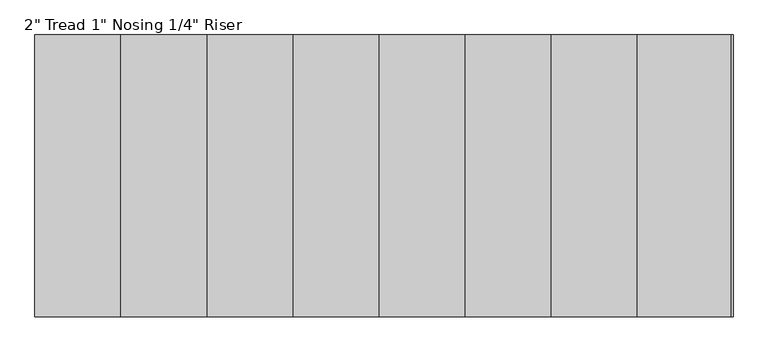
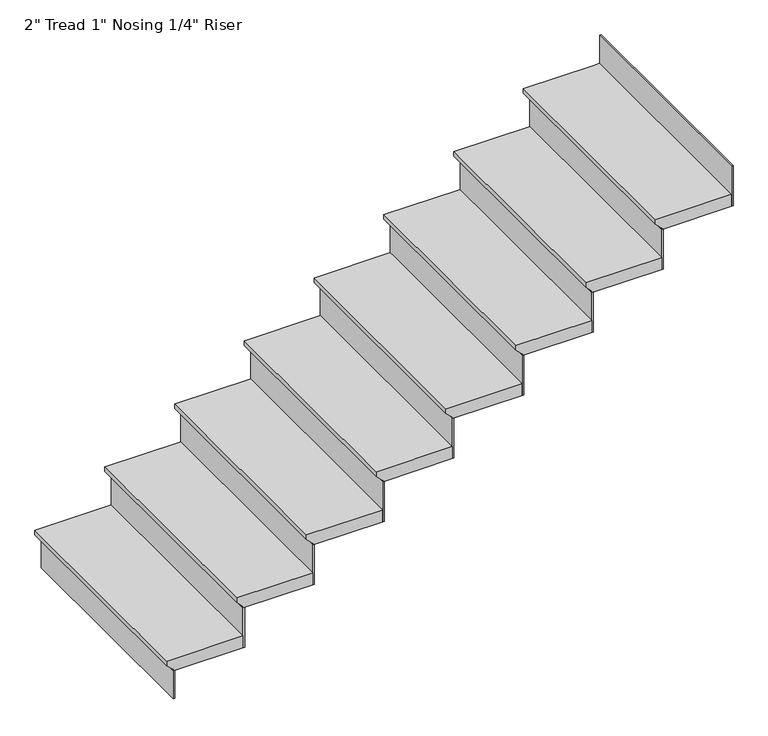
"""IFC4 building model written with IfcOpenShell, lengths in millimetres: stair flight geometry."""

from ifc_helpers import new_model, si_unit, origin, place, context, project, spatial, faceted_brep, source, transform, mapped, element, save


def stair_flight_5af034e0(model_context):
    return source(origin(), model_context, "Body", "Brep", [
        faceted_brep([(-4412.1017807, 444.1428136, 3350.6833333), (-4412.1017807, 444.1428136, 3369.7333333), (-4412.1017807, 1358.5428136, 3369.7333333), (-4412.1017807, 1358.5428136, 3350.6833333), (-4386.7017807, 444.1428136, 3325.2833333), (-4386.7017807, 1358.5428136, 3325.2833333), (-4107.3017807, 444.1428136, 3369.7333333), (-4107.3017807, 1358.5428136, 3369.7333333), (-4386.7017807, 1358.5428136, 3318.9333333), (-4107.3017807, 1358.5428136, 3318.9333333), (-4107.3017807, 444.1428136, 3318.9333333), (-4386.7017807, 444.1428136, 3318.9333333)], [[[0, 1, 2, 3]], [[4, 0, 3, 5]], [[2, 1, 6, 7]], [[8, 9, 10, 11]], [[2, 7, 9, 8, 5, 3]], [[8, 11, 4, 5]], [[6, 1, 0, 4, 11, 10]], [[7, 6, 10, 9]]]),
        faceted_brep([(-4386.7017807, 444.1428136, 3318.9333333), (-4386.7017807, 444.1428136, 3200.4), (-4380.3517807, 444.1428136, 3200.4), (-4380.3517807, 444.1428136, 3318.9333333), (-4386.7017807, 1358.5428136, 3318.9333333), (-4380.3517807, 1358.5428136, 3318.9333333), (-4380.3517807, 1358.5428136, 3200.4), (-4386.7017807, 1358.5428136, 3200.4)], [[[0, 1, 2, 3]], [[4, 5, 6, 7]], [[1, 0, 4, 7]], [[2, 1, 7, 6]], [[3, 2, 6, 5]], [[0, 3, 5, 4]]]),
        faceted_brep([(-4107.3017807, 444.1428136, 3488.2666667), (-4107.3017807, 444.1428136, 3318.9333333), (-4100.9517807, 444.1428136, 3318.9333333), (-4100.9517807, 444.1428136, 3488.2666667), (-4107.3017807, 1358.5428136, 3488.2666667), (-4100.9517807, 1358.5428136, 3488.2666667), (-4100.9517807, 1358.5428136, 3318.9333333), (-4107.3017807, 1358.5428136, 3318.9333333)], [[[0, 1, 2, 3]], [[4, 5, 6, 7]], [[1, 0, 4, 7]], [[2, 1, 7, 6]], [[3, 2, 6, 5]], [[0, 3, 5, 4]]]),
        faceted_brep([(-4132.7017807, 1358.5428136, 3539.0666667), (-4132.7017807, 444.1428136, 3539.0666667), (-3827.9017807, 444.1428136, 3539.0666667), (-3827.9017807, 1358.5428136, 3539.0666667), (-4107.3017807, 1358.5428136, 3488.2666667), (-3827.9017807, 1358.5428136, 3488.2666667), (-3827.9017807, 444.1428136, 3488.2666667), (-4107.3017807, 444.1428136, 3488.2666667), (-4107.3017807, 1358.5428136, 3494.6166667), (-4132.7017807, 1358.5428136, 3520.0166667), (-4107.3017807, 444.1428136, 3494.6166667), (-4132.7017807, 444.1428136, 3520.0166667)], [[[0, 1, 2, 3]], [[4, 5, 6, 7]], [[0, 3, 5, 4, 8, 9]], [[4, 7, 10, 8]], [[2, 1, 11, 10, 7, 6]], [[3, 2, 6, 5]], [[11, 1, 0, 9]], [[10, 11, 9, 8]]]),
        faceted_brep([(-3827.9017807, 444.1428136, 3657.6), (-3827.9017807, 444.1428136, 3488.2666667), (-3821.5517807, 444.1428136, 3488.2666667), (-3821.5517807, 444.1428136, 3657.6), (-3827.9017807, 1358.5428136, 3657.6), (-3821.5517807, 1358.5428136, 3657.6), (-3821.5517807, 1358.5428136, 3488.2666667), (-3827.9017807, 1358.5428136, 3488.2666667)], [[[0, 1, 2, 3]], [[4, 5, 6, 7]], [[1, 0, 4, 7]], [[2, 1, 7, 6]], [[3, 2, 6, 5]], [[0, 3, 5, 4]]]),
        faceted_brep([(-3853.3017807, 1358.5428136, 3708.4), (-3853.3017807, 444.1428136, 3708.4), (-3548.5017807, 444.1428136, 3708.4), (-3548.5017807, 1358.5428136, 3708.4), (-3827.9017807, 1358.5428136, 3657.6), (-3548.5017807, 1358.5428136, 3657.6), (-3548.5017807, 444.1428136, 3657.6), (-3827.9017807, 444.1428136, 3657.6), (-3827.9017807, 1358.5428136, 3663.95), (-3853.3017807, 1358.5428136, 3689.35), (-3827.9017807, 444.1428136, 3663.95), (-3853.3017807, 444.1428136, 3689.35)], [[[0, 1, 2, 3]], [[4, 5, 6, 7]], [[0, 3, 5, 4, 8, 9]], [[4, 7, 10, 8]], [[2, 1, 11, 10, 7, 6]], [[3, 2, 6, 5]], [[11, 1, 0, 9]], [[10, 11, 9, 8]]]),
        faceted_brep([(-3548.5017807, 444.1428136, 3826.9333333), (-3548.5017807, 444.1428136, 3657.6), (-3542.1517807, 444.1428136, 3657.6), (-3542.1517807, 444.1428136, 3826.9333333), (-3548.5017807, 1358.5428136, 3826.9333333), (-3542.1517807, 1358.5428136, 3826.9333333), (-3542.1517807, 1358.5428136, 3657.6), (-3548.5017807, 1358.5428136, 3657.6)], [[[0, 1, 2, 3]], [[4, 5, 6, 7]], [[1, 0, 4, 7]], [[2, 1, 7, 6]], [[3, 2, 6, 5]], [[0, 3, 5, 4]]]),
        faceted_brep([(-3573.9017807, 1358.5428136, 3877.7333333), (-3573.9017807, 444.1428136, 3877.7333333), (-3269.1017807, 444.1428136, 3877.7333333), (-3269.1017807, 1358.5428136, 3877.7333333), (-3548.5017807, 1358.5428136, 3826.9333333), (-3269.1017807, 1358.5428136, 3826.9333333), (-3269.1017807, 444.1428136, 3826.9333333), (-3548.5017807, 444.1428136, 3826.9333333), (-3548.5017807, 1358.5428136, 3833.2833333), (-3573.9017807, 1358.5428136, 3858.6833333), (-3548.5017807, 444.1428136, 3833.2833333), (-3573.9017807, 444.1428136, 3858.6833333)], [[[0, 1, 2, 3]], [[4, 5, 6, 7]], [[0, 3, 5, 4, 8, 9]], [[4, 7, 10, 8]], [[2, 1, 11, 10, 7, 6]], [[3, 2, 6, 5]], [[11, 1, 0, 9]], [[10, 11, 9, 8]]]),
        faceted_brep([(-3269.1017807, 444.1428136, 3996.2666667), (-3269.1017807, 444.1428136, 3826.9333333), (-3262.7517807, 444.1428136, 3826.9333333), (-3262.7517807, 444.1428136, 3996.2666667), (-3269.1017807, 1358.5428136, 3996.2666667), (-3262.7517807, 1358.5428136, 3996.2666667), (-3262.7517807, 1358.5428136, 3826.9333333), (-3269.1017807, 1358.5428136, 3826.9333333)], [[[0, 1, 2, 3]], [[4, 5, 6, 7]], [[1, 0, 4, 7]], [[2, 1, 7, 6]], [[3, 2, 6, 5]], [[0, 3, 5, 4]]]),
        faceted_brep([(-3294.5017807, 1358.5428136, 4047.0666667), (-3294.5017807, 444.1428136, 4047.0666667), (-2989.7017807, 444.1428136, 4047.0666667), (-2989.7017807, 1358.5428136, 4047.0666667), (-3269.1017807, 1358.5428136, 3996.2666667), (-2989.7017807, 1358.5428136, 3996.2666667), (-2989.7017807, 444.1428136, 3996.2666667), (-3269.1017807, 444.1428136, 3996.2666667), (-3269.1017807, 1358.5428136, 4002.6166667), (-3294.5017807, 1358.5428136, 4028.0166667), (-3269.1017807, 444.1428136, 4002.6166667), (-3294.5017807, 444.1428136, 4028.0166667)], [[[0, 1, 2, 3]], [[4, 5, 6, 7]], [[0, 3, 5, 4, 8, 9]], [[4, 7, 10, 8]], [[2, 1, 11, 10, 7, 6]], [[3, 2, 6, 5]], [[11, 1, 0, 9]], [[10, 11, 9, 8]]]),
        faceted_brep([(-2989.7017807, 444.1428136, 4165.6), (-2989.7017807, 444.1428136, 3996.2666667), (-2983.3517807, 444.1428136, 3996.2666667), (-2983.3517807, 444.1428136, 4165.6), (-2989.7017807, 1358.5428136, 4165.6), (-2983.3517807, 1358.5428136, 4165.6), (-2983.3517807, 1358.5428136, 3996.2666667), (-2989.7017807, 1358.5428136, 3996.2666667)], [[[0, 1, 2, 3]], [[4, 5, 6, 7]], [[1, 0, 4, 7]], [[2, 1, 7, 6]], [[3, 2, 6, 5]], [[0, 3, 5, 4]]]),
        faceted_brep([(-3015.1017807, 1358.5428136, 4216.4), (-3015.1017807, 444.1428136, 4216.4), (-2710.3017807, 444.1428136, 4216.4), (-2710.3017807, 1358.5428136, 4216.4), (-2989.7017807, 1358.5428136, 4165.6), (-2710.3017807, 1358.5428136, 4165.6), (-2710.3017807, 444.1428136, 4165.6), (-2989.7017807, 444.1428136, 4165.6), (-2989.7017807, 1358.5428136, 4171.95), (-3015.1017807, 1358.5428136, 4197.35), (-2989.7017807, 444.1428136, 4171.95), (-3015.1017807, 444.1428136, 4197.35)], [[[0, 1, 2, 3]], [[4, 5, 6, 7]], [[0, 3, 5, 4, 8, 9]], [[4, 7, 10, 8]], [[2, 1, 11, 10, 7, 6]], [[3, 2, 6, 5]], [[11, 1, 0, 9]], [[10, 11, 9, 8]]]),
        faceted_brep([(-2710.3017807, 444.1428136, 4334.9333333), (-2710.3017807, 444.1428136, 4165.6), (-2703.9517807, 444.1428136, 4165.6), (-2703.9517807, 444.1428136, 4334.9333333), (-2710.3017807, 1358.5428136, 4334.9333333), (-2703.9517807, 1358.5428136, 4334.9333333), (-2703.9517807, 1358.5428136, 4165.6), (-2710.3017807, 1358.5428136, 4165.6)], [[[0, 1, 2, 3]], [[4, 5, 6, 7]], [[1, 0, 4, 7]], [[2, 1, 7, 6]], [[3, 2, 6, 5]], [[0, 3, 5, 4]]]),
        faceted_brep([(-2735.7017807, 1358.5428136, 4385.7333333), (-2735.7017807, 444.1428136, 4385.7333333), (-2430.9017807, 444.1428136, 4385.7333333), (-2430.9017807, 1358.5428136, 4385.7333333), (-2710.3017807, 1358.5428136, 4334.9333333), (-2430.9017807, 1358.5428136, 4334.9333333), (-2430.9017807, 444.1428136, 4334.9333333), (-2710.3017807, 444.1428136, 4334.9333333), (-2710.3017807, 1358.5428136, 4341.2833333), (-2735.7017807, 1358.5428136, 4366.6833333), (-2710.3017807, 444.1428136, 4341.2833333), (-2735.7017807, 444.1428136, 4366.6833333)], [[[0, 1, 2, 3]], [[4, 5, 6, 7]], [[0, 3, 5, 4, 8, 9]], [[4, 7, 10, 8]], [[2, 1, 11, 10, 7, 6]], [[3, 2, 6, 5]], [[11, 1, 0, 9]], [[10, 11, 9, 8]]]),
        faceted_brep([(-2151.5017807, 444.1428136, 4673.6), (-2151.5017807, 444.1428136, 4504.2666667), (-2145.1517807, 444.1428136, 4504.2666667), (-2145.1517807, 444.1428136, 4673.6), (-2151.5017807, 1358.5428136, 4673.6), (-2145.1517807, 1358.5428136, 4673.6), (-2145.1517807, 1358.5428136, 4504.2666667), (-2151.5017807, 1358.5428136, 4504.2666667)], [[[0, 1, 2, 3]], [[4, 5, 6, 7]], [[1, 0, 4, 7]], [[2, 1, 7, 6]], [[3, 2, 6, 5]], [[0, 3, 5, 4]]]),
        faceted_brep([(-2430.9017807, 444.1428136, 4504.2666667), (-2430.9017807, 444.1428136, 4334.9333333), (-2424.5517807, 444.1428136, 4334.9333333), (-2424.5517807, 444.1428136, 4504.2666667), (-2430.9017807, 1358.5428136, 4504.2666667), (-2424.5517807, 1358.5428136, 4504.2666667), (-2424.5517807, 1358.5428136, 4334.9333333), (-2430.9017807, 1358.5428136, 4334.9333333)], [[[0, 1, 2, 3]], [[4, 5, 6, 7]], [[1, 0, 4, 7]], [[2, 1, 7, 6]], [[3, 2, 6, 5]], [[0, 3, 5, 4]]]),
        faceted_brep([(-2151.5017807, 1358.5428136, 4555.0666667), (-2176.9017807, 1358.5428136, 4555.0666667), (-2456.3017807, 1358.5428136, 4555.0666667), (-2456.3017807, 444.1428136, 4555.0666667), (-2151.5017807, 444.1428136, 4555.0666667), (-2176.9017807, 1358.5428136, 4504.2666667), (-2151.5017807, 1358.5428136, 4504.2666667), (-2151.5017807, 444.1428136, 4504.2666667), (-2430.9017807, 444.1428136, 4504.2666667), (-2430.9017807, 1358.5428136, 4504.2666667), (-2430.9017807, 1358.5428136, 4510.6166667), (-2456.3017807, 1358.5428136, 4536.0166667), (-2430.9017807, 444.1428136, 4510.6166667), (-2456.3017807, 444.1428136, 4536.0166667)], [[[0, 1, 2, 3, 4]], [[5, 6, 7, 8, 9]], [[1, 0, 6, 5]], [[2, 1, 5, 9, 10, 11]], [[9, 8, 12, 10]], [[4, 3, 13, 12, 8, 7]], [[0, 4, 7, 6]], [[13, 3, 2, 11]], [[12, 13, 11, 10]]]),
    ])


if __name__ == "__main__":
    model = new_model("IFC4")
    model_context = context("Model", 3, world=origin())
    ifc_project = project(units=[si_unit("LENGTHUNIT", "METRE", prefix="MILLI")], contexts=[model_context])
    site = spatial("IfcSite", under=ifc_project)
    building = spatial("IfcBuilding", under=site)
    placement = place(None, origin())
    stair_flight_shape = stair_flight_5af034e0(model_context)
    element("IfcStairFlight", 1, ObjectType="2\" Tread 1\" Nosing 1/4\" Riser", at=placement, inside=building, context=model_context, shape_type="MappedRepresentation", body=[
        mapped(stair_flight_shape, transform((0.0, 0.0, 0.0), x_axis=(1.0, 0.0, 0.0), y_axis=(0.0, 1.0, 0.0), z_axis=(0.0, 0.0, 1.0))),
    ])
    save(model, "model.ifc")
